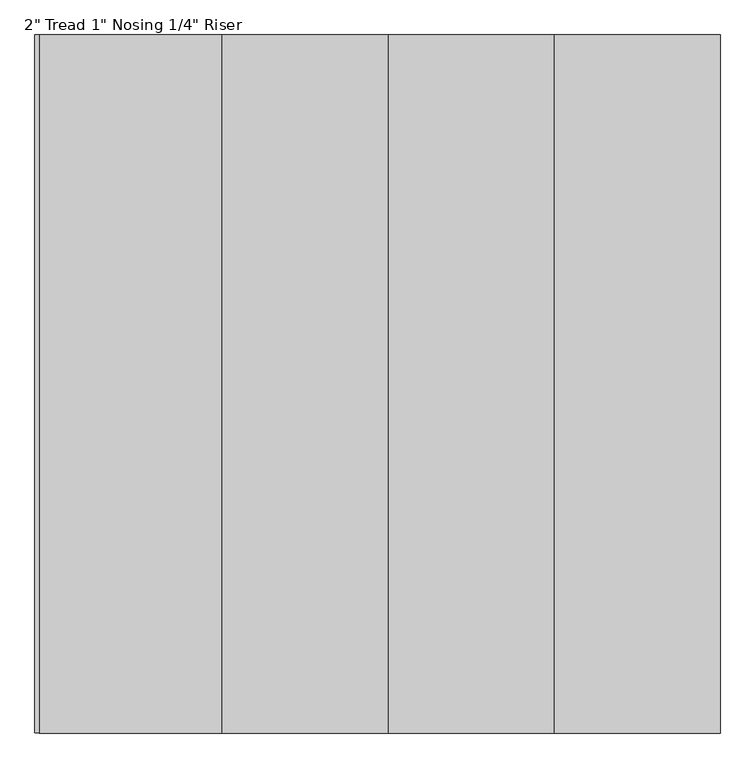
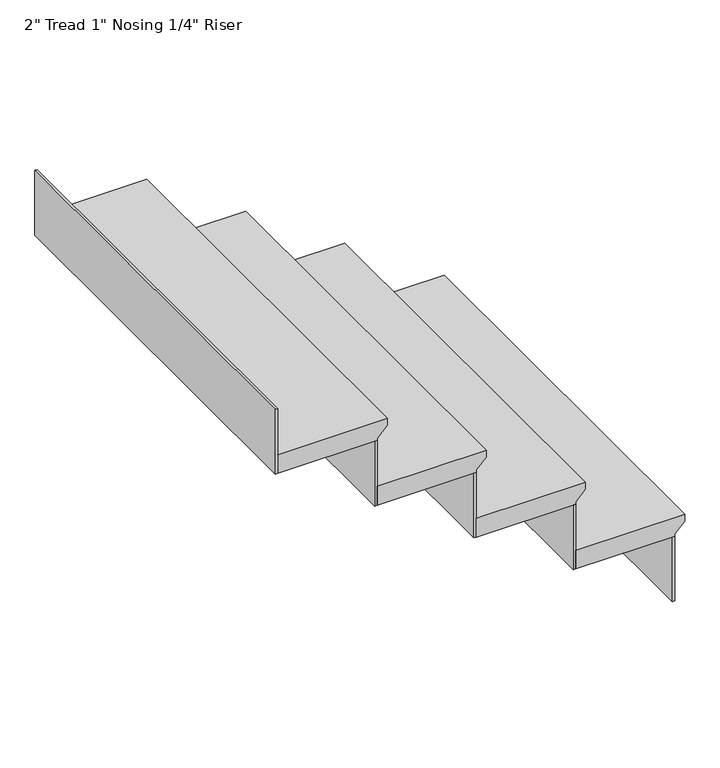
"""IFC4 building model written with IfcOpenShell, lengths in millimetres: stair flight geometry."""

from ifc_helpers import new_model, si_unit, frame, origin, place, context, project, spatial, polyline, outline, extrude, source, transform, mapped, element, save


def stair_flight_f733f96e(model_context):
    return source(origin(), model_context, "Body", "SweptSolid", [
        extrude(outline(polyline([(2804.16, 17678.7916032), (2804.16, 17399.3916032), (2753.36, 17399.3916032), (2753.36, 17653.3916032), (2759.71, 17653.3916032), (2785.11, 17678.7916032), (2804.16, 17678.7916032)])), frame((0.0, 1802.3241878, 0.0), z_axis=(0.0, 1.0, 0.0), x_axis=(0.0, 0.0, 1.0)), (0.0, 0.0, 1.0), 1066.8),
        extrude(outline(polyline([(17647.0416032, 2869.1241878), (17653.3916032, 2869.1241878), (17653.3916032, 1802.3241878), (17647.0416032, 1802.3241878), (17647.0416032, 2869.1241878)])), frame((0.0, 0.0, 2578.1), z_axis=(0.0, 0.0, 1.0), x_axis=(1.0, 0.0, 0.0)), (0.0, 0.0, 1.0), 175.26),
        extrude(outline(polyline([(17393.0416032, 2869.1241878), (17399.3916032, 2869.1241878), (17399.3916032, 1802.3241878), (17393.0416032, 1802.3241878), (17393.0416032, 2869.1241878)])), frame((0.0, 0.0, 2753.36), z_axis=(0.0, 0.0, 1.0), x_axis=(1.0, 0.0, 0.0)), (0.0, 0.0, 1.0), 175.26),
        extrude(outline(polyline([(2979.42, 17424.7916032), (2979.42, 17145.3916032), (2928.62, 17145.3916032), (2928.62, 17399.3916032), (2934.97, 17399.3916032), (2960.37, 17424.7916032), (2979.42, 17424.7916032)])), frame((0.0, 1802.3241878, 0.0), z_axis=(0.0, 1.0, 0.0), x_axis=(0.0, 0.0, 1.0)), (0.0, 0.0, 1.0), 1066.8),
        extrude(outline(polyline([(17139.0416032, 2869.1241878), (17145.3916032, 2869.1241878), (17145.3916032, 1802.3241878), (17139.0416032, 1802.3241878), (17139.0416032, 2869.1241878)])), frame((0.0, 0.0, 2928.62), z_axis=(0.0, 0.0, 1.0), x_axis=(1.0, 0.0, 0.0)), (0.0, 0.0, 1.0), 175.26),
        extrude(outline(polyline([(3154.68, 17170.7916032), (3154.68, 16891.3916032), (3103.88, 16891.3916032), (3103.88, 17145.3916032), (3110.23, 17145.3916032), (3135.63, 17170.7916032), (3154.68, 17170.7916032)])), frame((0.0, 1802.3241878, 0.0), z_axis=(0.0, 1.0, 0.0), x_axis=(0.0, 0.0, 1.0)), (0.0, 0.0, 1.0), 1066.8),
        extrude(outline(polyline([(16885.0416032, 2869.1241878), (16891.3916032, 2869.1241878), (16891.3916032, 1802.3241878), (16885.0416032, 1802.3241878), (16885.0416032, 2869.1241878)])), frame((0.0, 0.0, 3103.88), z_axis=(0.0, 0.0, 1.0), x_axis=(1.0, 0.0, 0.0)), (0.0, 0.0, 1.0), 175.26),
        extrude(outline(polyline([(16631.0416032, 2869.1241878), (16637.3916032, 2869.1241878), (16637.3916032, 1802.3241878), (16631.0416032, 1802.3241878), (16631.0416032, 2869.1241878)])), frame((0.0, 0.0, 3279.14), z_axis=(0.0, 0.0, 1.0), x_axis=(1.0, 0.0, 0.0)), (0.0, 0.0, 1.0), 175.26),
        extrude(outline(polyline([(3329.94, 16916.7916032), (3329.94, 16637.3916032), (3279.14, 16637.3916032), (3279.14, 16891.3916032), (3285.49, 16891.3916032), (3310.89, 16916.7916032), (3329.94, 16916.7916032)])), frame((0.0, 1802.3241878, 0.0), z_axis=(0.0, 1.0, 0.0), x_axis=(0.0, 0.0, 1.0)), (0.0, 0.0, 1.0), 1066.8),
    ])


if __name__ == "__main__":
    model = new_model("IFC4")
    model_context = context("Model", 3, world=origin())
    ifc_project = project(units=[si_unit("LENGTHUNIT", "METRE", prefix="MILLI")], contexts=[model_context])
    site = spatial("IfcSite", under=ifc_project)
    building = spatial("IfcBuilding", under=site)
    placement = place(None, origin())
    stair_flight_shape = stair_flight_f733f96e(model_context)
    element("IfcStairFlight", 1, ObjectType="2\" Tread 1\" Nosing 1/4\" Riser", at=placement, inside=building, context=model_context, shape_type="MappedRepresentation", body=[
        mapped(stair_flight_shape, transform((0.0, 0.0, 0.0), x_axis=(1.0, 0.0, 0.0), y_axis=(0.0, 1.0, 0.0), z_axis=(0.0, 0.0, 1.0))),
    ])
    save(model, "model.ifc")
